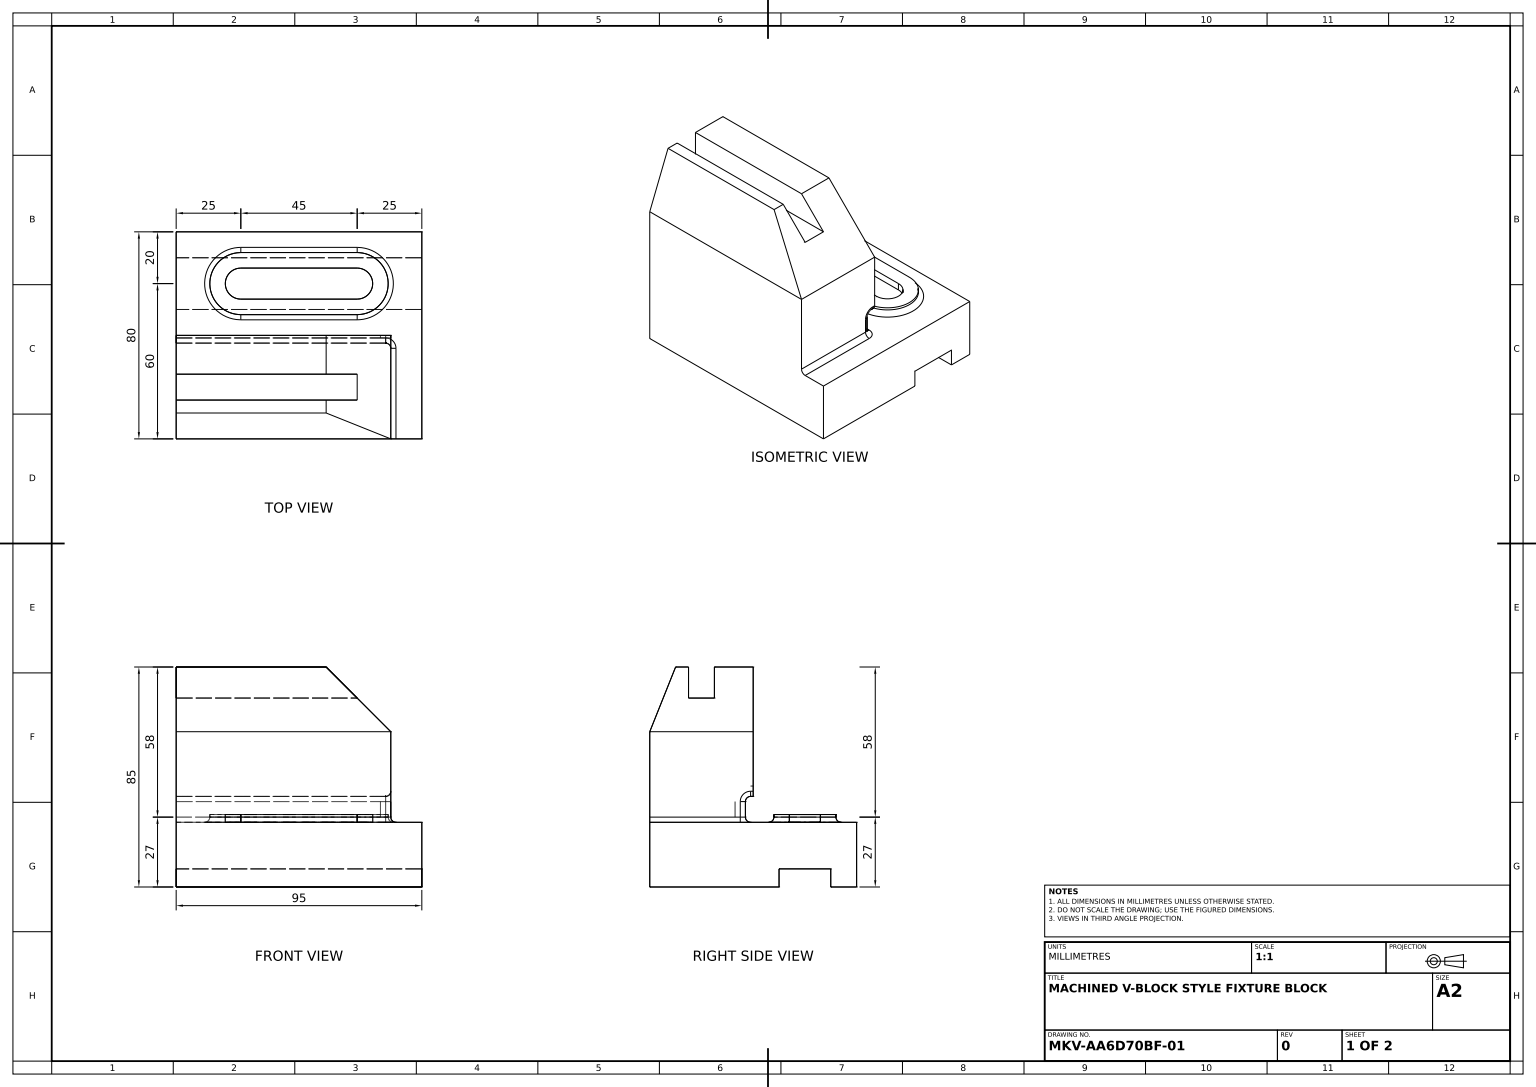
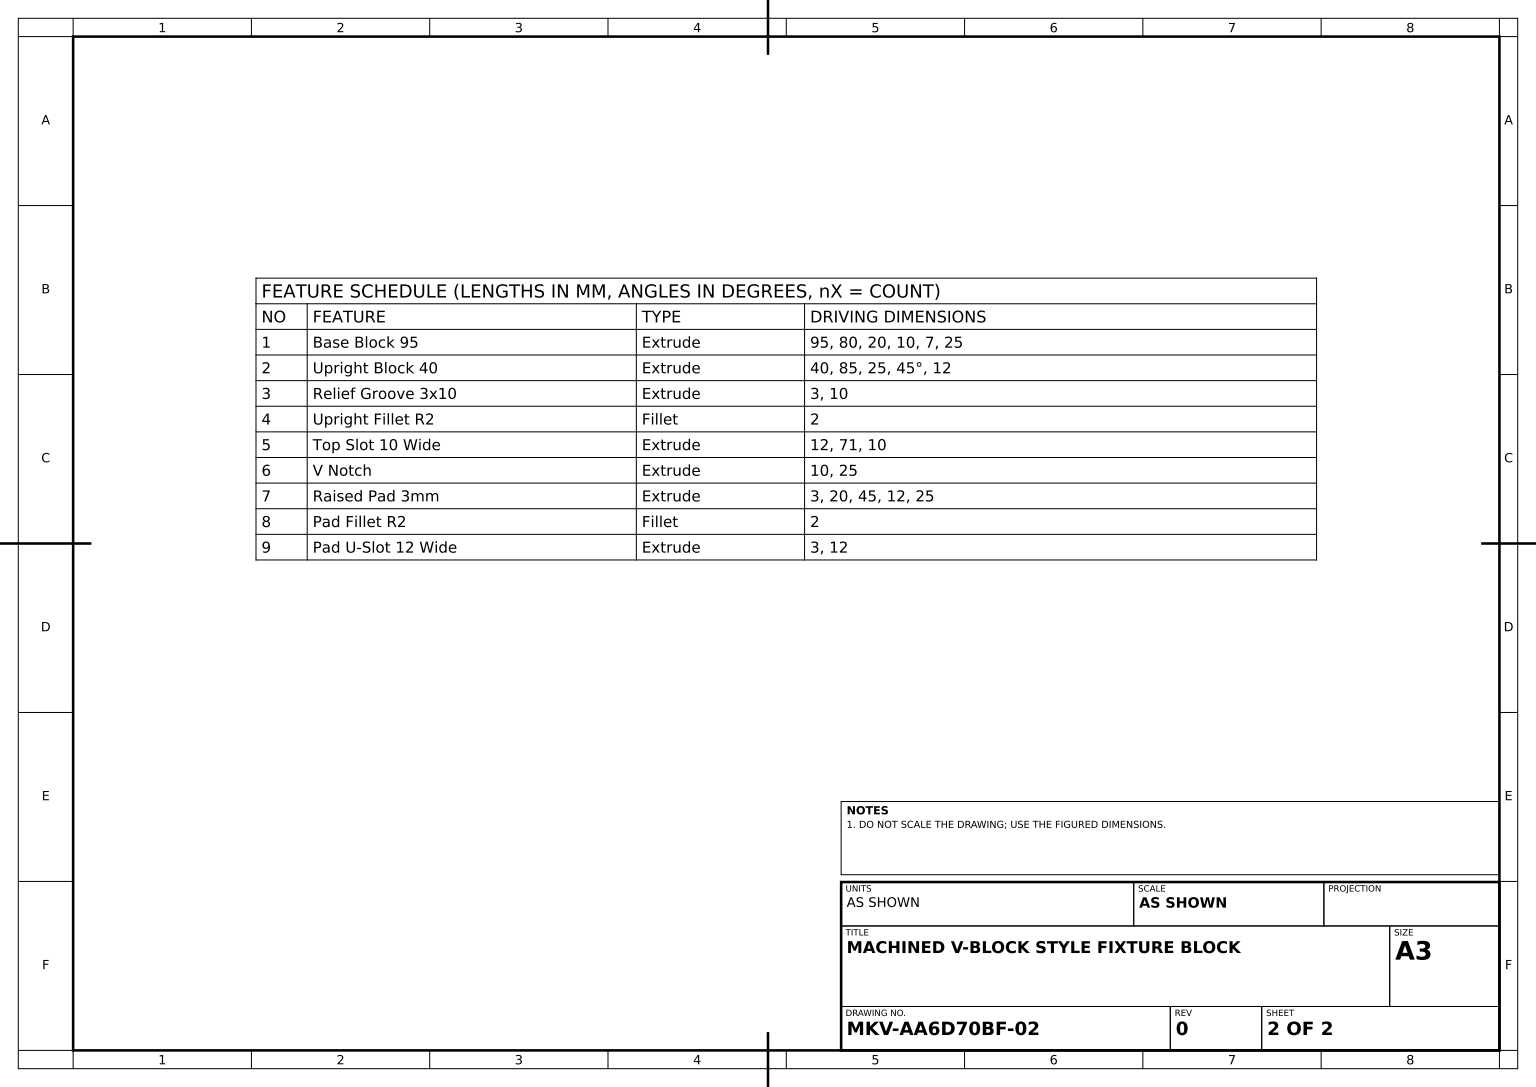
SolidWorks part; units mm, degrees
material "Plain Carbon Steel"
ref_plane "Front Plane" through (0, 0, 0) normal (0, 0, 1) x (1, 0, 0)
ref_plane "Top Plane" through (0, 0, 0) normal (0, 1, 0) x (1, 0, 0)
ref_plane "Right Plane" through (0, 0, 0) normal (1, 0, 0) x (0, 0, -1)
sketch "Base Profile Sketch" plane through (0, 0, 0) normal (1, 0, 0) x (0, 0, -1)
  line L0 (0, 0) -> (50, 0)
  line L1 (50, 0) -> (50, 7)
  line L2 (50, 7) -> (70, 7)
  line L3 (70, 7) -> (70, 0)
  line L4 (70, 0) -> (80, 0)
  line L5 (80, 0) -> (80, 25)
  line L6 (80, 25) -> (0, 25)
  line L7 (0, 25) -> (0, 0)
  dimension "D1" = 80
  dimension "D2" = 20
  dimension "D3" = 10
  dimension "D4" = 7
  dimension "D5" = 25
extrude "Base Block 95" add sketch "Base Profile Sketch" along normal mid plane 95
sketch "Upright Profile Sketch" plane through (0, 0, 0) normal (0, 0, 1) x (1, 0, 0)
  line L0 (-47.5, 25) -> (-47.5, 85)
  line L1 (-47.5, 85) -> (10.5, 85)
  line L2 (10.5, 85) -> (35.5, 60)
  line L3 (35.5, 60) -> (35.5, 25)
  line L4 (47.5, 25) -> (-47.5, 25) construction
  line L5 (35.5, 25) -> (-47.5, 25)
  line L6 (47.5, 0) -> (-47.5, 0) construction
  line L7 (35.5, 60) -> (-30.3564, 60) construction
  line L9 (47.5, 25) -> (47.5, 0) construction
  dimension "D1" = 85
  dimension "D2" = 12
  dimension "D3" = 25
  dimension "D4" = 45
extrude "Upright Block 40" add sketch "Upright Profile Sketch" against normal blind 40
sketch "Relief Groove Sketch" plane through (35.5, 0, 0) normal (1, 0, 0) x (0, 0, -1)
  line L0 (40, 35) -> (37, 35)
  line L1 (40, 25) -> (40, 60) construction
  line L2 (37, 35) -> (37, 25)
  line L3 (40, 25) -> (0, 25) construction
  line L4 (37, 25) -> (40, 25)
  line L5 (80, 25) -> (0, 25) construction
  line L6 (40, 25) -> (40, 35)
  dimension "D1" = 3
  dimension "D2" = 10
extrude "Relief Groove 3x10" cut sketch "Relief Groove Sketch" against normal through all contours L0 L2 L4 L6
fillet "Upright Fillet R2" radius 2 5 edges at (35.5, 35, -38.5) (-6, 35, -37) (35.5, 30, -37) (-6, 25, -37) (35.5, 25, -18.5)
sketch "Top Slot Sketch" plane through (0, 85, 0) normal (0, 1, 0) x (1, 0, 0)
  line L0 (-47.5, 20) -> (51.5432, 20) construction
  line L1 (-47.5, 40) -> (-47.5, 0) construction
  line L5 (-47.5, 15) -> (23.5, 15)
  line L6 (-47.5, 15) -> (-47.5, 25)
  line L7 (-47.5, 25) -> (23.5, 25)
  line L8 (23.5, 15) -> (23.5, 25)
  point P9 (-47.5, 20)
  dimension "D1" = 71
  dimension "D2" = 10
extrude "Top Slot 10 Wide" cut sketch "Top Slot Sketch" against normal blind 12 contours L7 L8 L5 L6
sketch "V Notch Sketch" plane through (-47.5, 0, 0) normal (-1, 0, 0) x (0, 0, 1)
  line L0 (0, 60) -> (0, 85)
  line L1 (0, 85) -> (0, 0) construction
  line L2 (0, 85) -> (-10, 85)
  line L3 (-15, 85) -> (0, 85) construction
  line L4 (-10, 85) -> (0, 60)
  dimension "D1" = 10
  dimension "D2" = 25
extrude "V Notch" cut sketch "V Notch Sketch" against normal through all
sketch "Raised Pad Sketch" plane through (0, 25, 0) normal (0, 1, 0) x (1, 0, 0)
  line L0 (-22.5, 60) -> (22.5, 60) construction
  line L1 (-22.5, 72) -> (22.5, 72)
  line L2 (-22.5, 48) -> (22.5, 48)
  line L3 (47.5, 80) -> (-47.5, 80) construction
  line L4 (47.5, 80) -> (47.5, 0) construction
  arc A0 (-22.5, 72) -> (-22.5, 48) centre (-22.5, 60) ccw
  arc A1 (22.5, 48) -> (22.5, 72) centre (22.5, 60) ccw
  point P2 (0, 60)
  dimension "D3" = 12
  dimension "D1" = 20
  dimension "D2" = 45
  dimension "D4" = 25
extrude "Raised Pad 3mm" add sketch "Raised Pad Sketch" along normal blind 3
fillet "Pad Fillet R2" radius 2 4 edges at (34.5, 25, -60) (0, 25, -48) (-34.5, 25, -60) (0, 25, -72)
sketch "Pad Slot Sketch" plane through (0, 28, 0) normal (0, 1, 0) x (1, 0, 0)
  line L0 (-22.5, 60) -> (22.5, 60) construction
  line L1 (-22.5, 66) -> (22.5, 66)
  line L2 (-22.5, 54) -> (22.5, 54)
  arc A0 (-22.5, 66) -> (-22.5, 54) centre (-22.5, 60) ccw
  arc A1 (22.5, 54) -> (22.5, 66) centre (22.5, 60) ccw
  point P4 (0, 60)
  dimension "D1" = 12
extrude "Pad U-Slot 12 Wide" cut sketch "Pad Slot Sketch" against normal blind 3
